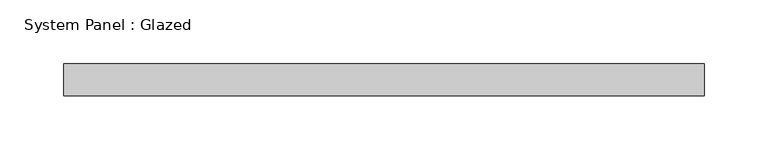
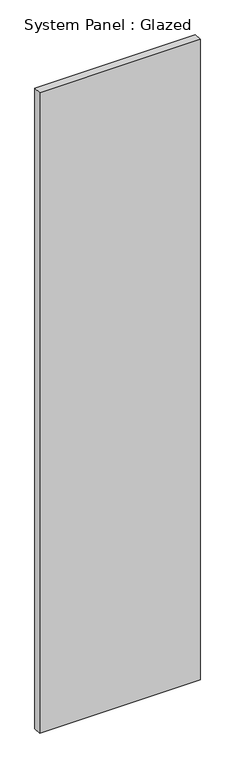
"""IFC4 building model written with IfcOpenShell, lengths in millimetres: plate geometry, System Panel : Glazed."""

from ifc_helpers import new_model, si_unit, origin, origin_with_axes, place, context, project, spatial, polyline, outline, extrude, source, transform, mapped, element, save


def system_panel_glazed_7695abb4(model_context):
    return source(origin(), model_context, "Body", "SweptSolid", [
        extrude(outline(polyline([(251.25, 24.5), (-251.25, 24.5), (-251.25, 49.5), (251.25, 49.5), (251.25, 24.5)])), origin_with_axes(), (0.0, 0.0, 1.0), 2120.0),
    ])


if __name__ == "__main__":
    model = new_model("IFC4")
    model_context = context("Model", 3, world=origin())
    ifc_project = project(units=[si_unit("LENGTHUNIT", "METRE", prefix="MILLI")], contexts=[model_context])
    site = spatial("IfcSite", under=ifc_project)
    building = spatial("IfcBuilding", under=site)
    placement = place(None, origin())
    system_panel_glazed_shape = system_panel_glazed_7695abb4(model_context)
    element("IfcPlate", 1, ObjectType="System Panel : Glazed", at=placement, inside=building, context=model_context, shape_type="MappedRepresentation", body=[
        mapped(system_panel_glazed_shape, transform((0.0, 0.0, 0.0), x_axis=(1.0, 0.0, 0.0), y_axis=(0.0, 1.0, 0.0), z_axis=(0.0, 0.0, 1.0))),
    ])
    save(model, "model.ifc")

# Revit data of these elements
# Type "System Panel : Glazed"
#   Construction Type Id = "GSP4R"
#   Analytic Construction = "1/8 in Pilkington single glazing"
#   Visual Light Transmittance = 0.9
#   Solar Heat Gain Coefficient = 0.86
#   Heat Transfer Coefficient (U) = 6.7069 W/(m²·K)
#   Define Thermal Properties by = 1
# Element 1 (IfcPlate, "System Panel : Glazed")
#   Materials on its faces: "Glass"
# Materials
#   "Glass": class "Glass", colour RGB 245 245 243, transparency 1, Description = "Soda Lime Glass", Cost = 0
